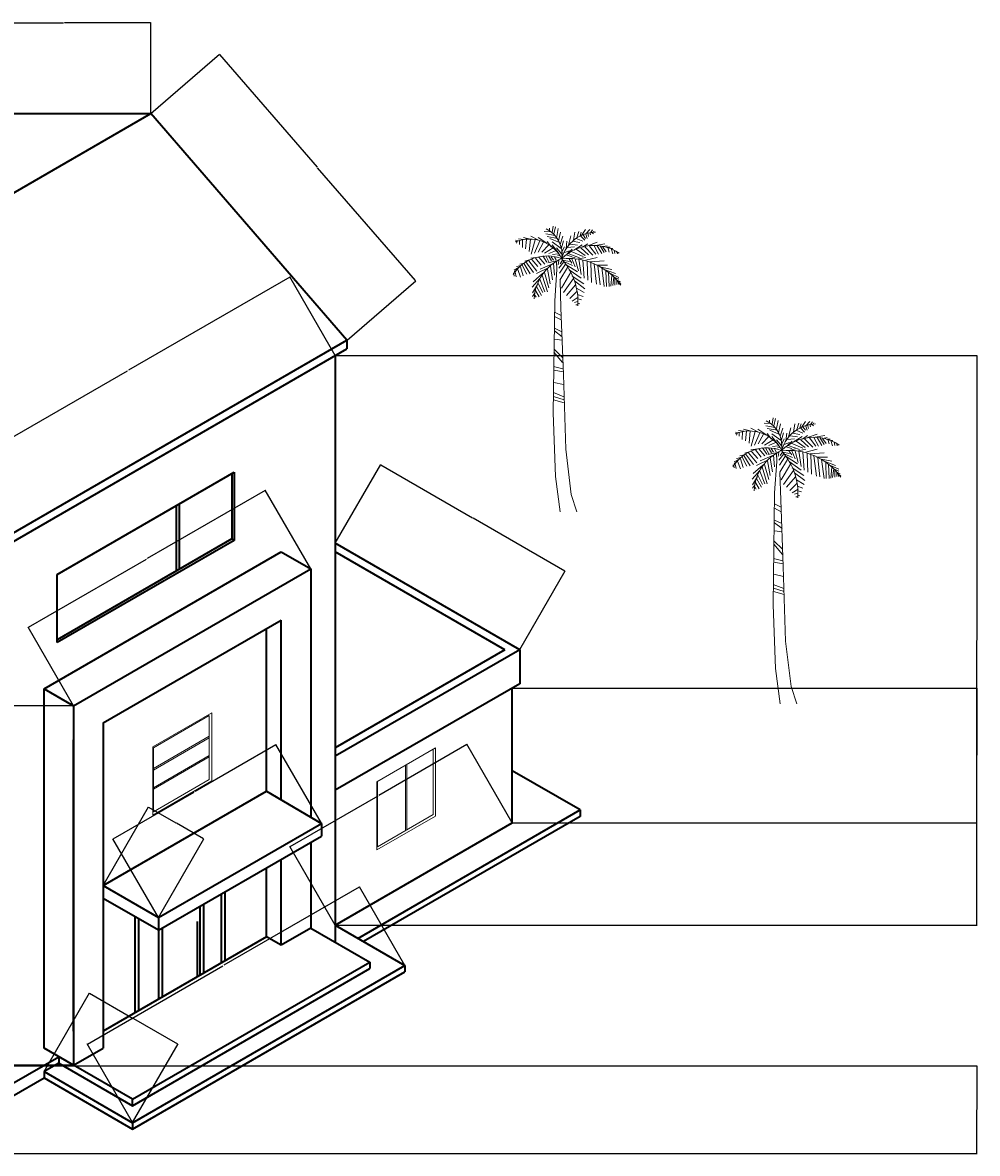
# Model space of a CAD drawing. Units: inches. Extents: x 159268 to 319465, y 115871 to 232488.
# Tile 2 of 2: x 159989 to 160662, y 116007 to 116803. Entities that reach past the tile are written whole.
import ezdxf

# ---------------------------------------------------------------- set-up
doc = ezdxf.new("R2010")
doc.units = ezdxf.units.IN
for name, color, linetype, lineweight in [('A-ANNO-DIMS', 2, 'Continuous', 18), ('A-ELEV', 7, 'Continuous', 35), ('A-GLAZ', 4, 'Continuous', 18), ('L-PLNT', 3, 'Continuous', 13)]:
    doc.layers.add(name, color=color, linetype=linetype, lineweight=lineweight)
doc.styles.get("Standard").update_dxf_attribs({"font": 'arial.ttf'})
doc.dimstyles.get("Standard").update_dxf_attribs({"dimtxt": 0.18, "dimasz": 0.18, "dimexe": 0.18, "dimexo": 0.0625, "dimgap": 0.09, "dimtad": 0, "dimtih": 1, "dimtoh": 1, "dimdec": 4, "dimzin": 0, "dimdsep": 46, "dimtxsty": 'Standard', "dimcen": 0.09, "dimadec": 0, "dimazin": 0, "dimtfac": 1, "dimtdec": 4, "dimtofl": 0, "dimtmove": 0, "dimatfit": 3, "dimfxl": 1, "dimtolj": 1, "dimtzin": 0, "dimarcsym": 0})

# ---------------------------------------------------------------- blocks, each defined once
blk = doc.blocks.new('*U5')
for p, q in [((-7.5, 199.68), (-7.5, 197.946)), ((-5.567, 196.707), (-4.987, 201.167)), ((-4.407, 195.716), (-3.247, 200.672)), ((-2.474, 193.733), (-1.315, 199.433)), ((-29.729, 190.759), (-31.469, 191.255)), ((-25.283, 191.751), (-29.342, 192.246)), ((-26.443, 191.503), (-26.636, 186.051)), ((-20.064, 191.751), (-25.863, 193.238)), ((-23.737, 191.751), (-24.51, 185.06)), ((-21.031, 191.998), (-21.804, 183.325)), ((-15.232, 191.255), (-20.644, 193.981)), ((-17.551, 191.503), (-20.451, 181.343)), ((-9.433, 189.025), (-15.618, 193.238)), ((-6.727, 197.202), (-11.366, 197.45)), ((-3.441, 194.477), (-10.013, 195.716)), ((-1.894, 192.494), (-9.24, 193.733)), ((-0.541, 189.52), (-7.307, 192.494)), ((-1.121, 190.759), (0.232, 196.955)), ((0.038, 188.281), (1.778, 193.981)), ((5.837, 187.786), (7.577, 194.229)), ((9.317, 191.255), (10.283, 196.955)), ((11.25, 192.494), (15.889, 190.512)), ((11.829, 192.99), (13.182, 197.45)), ((13.956, 194.229), (14.729, 196.955)), ((14.536, 193.981), (17.242, 191.255)), ((15.116, 194.477), (17.822, 198.689)), ((16.082, 194.972), (17.822, 192.494)), ((18.015, 195.716), (20.914, 198.689)), ((18.015, 195.468), (18.981, 192.494)), ((19.368, 196.459), (19.948, 193.733)), ((20.914, 196.459), (21.301, 194.972)), ((21.301, 196.459), (22.847, 198.441)), ((22.074, 196.707), (23.427, 195.716)), ((23.234, 196.707), (23.62, 197.698)), ((-30.309, 190.512), (-30.695, 189.025)), ((-28.763, 190.759), (-28.763, 188.281)), ((-14.265, 190.759), (-18.131, 182.086)), ((-11.753, 189.768), (-15.425, 182.83)), ((-8.08, 188.034), (-12.912, 182.83)), ((-4.987, 185.803), (-10.979, 182.086)), ((-6.147, 186.299), (-9.24, 190.264)), ((-3.247, 183.821), (-8.08, 181.838)), ((-5.76, 190.016), (0.618, 185.308)), ((-5.76, 188.034), (-1.508, 182.582)), ((-2.668, 185.803), (1.198, 181.343)), ((1.005, 185.803), (2.358, 190.759)), ((1.005, 182.582), (2.938, 186.547)), ((2.938, 182.582), (6.61, 183.821)), ((4.098, 185.06), (4.678, 190.512)), ((4.871, 186.051), (10.09, 186.547)), ((4.871, 181.591), (8.544, 184.812)), ((6.997, 188.529), (12.216, 187.786)), ((7.77, 183.325), (16.082, 179.856)), ((8.544, 190.512), (13.763, 189.52)), ((9.51, 184.317), (15.502, 188.034)), ((11.25, 184.812), (17.628, 180.352)), ((14.536, 185.803), (19.948, 180.847)), ((15.695, 186.299), (19.368, 188.777)), ((17.242, 186.547), (23.041, 180.599)), ((19.368, 187.29), (26.133, 189.768)), ((20.721, 187.042), (25.167, 181.343)), ((23.814, 187.29), (26.907, 181.343)), ((24.78, 187.538), (31.546, 188.777)), ((26.133, 187.29), (29.419, 181.838)), ((28.066, 187.29), (30.966, 182.582)), ((29.806, 186.795), (32.319, 183.078)), ((29.999, 186.795), (33.092, 187.29)), ((32.512, 186.299), (35.218, 186.299)), ((33.479, 186.051), (34.445, 182.83)), ((35.605, 185.556), (37.151, 185.308)), ((35.798, 185.308), (36.958, 181.591)), ((38.118, 184.317), (38.504, 181.838)), ((-25.09, 175.148), (-28.376, 174.404)), ((-21.031, 177.626), (-24.897, 176.387)), ((-24.317, 175.891), (-18.711, 168.457)), ((-22.191, 176.635), (-16.391, 169.448)), ((-15.618, 179.36), (-20.644, 178.617)), ((-20.064, 177.626), (-15.812, 172.67)), ((-17.358, 178.617), (-13.299, 173.661)), ((-15.038, 179.36), (-10.786, 174.404)), ((-4.214, 175.148), (-14.072, 170.935)), ((-12.332, 180.104), (-9.433, 175.643)), ((-10.206, 180.104), (-8.08, 175.891)), ((-1.701, 176.882), (-8.66, 175.396)), ((-8.273, 180.104), (-6.147, 176.635)), ((-6.34, 179.608), (-4.6, 177.13)), ((-1.315, 181.591), (-5.374, 181.095)), ((-4.021, 179.36), (-2.861, 177.378)), ((-2.668, 176.387), (-2.376, 170.594)), ((-0.348, 180.352), (-1.894, 180.104)), ((-0.928, 176.882), (-1.508, 173.909)), ((2.551, 175.891), (-0.928, 171.431)), ((1.585, 177.13), (0.038, 174.652)), ((1.585, 177.13), (6.61, 176.139)), ((2.938, 175.891), (8.737, 173.413)), ((4.098, 180.847), (8.35, 179.608)), ((5.644, 181.838), (13.569, 178.865)), ((6.224, 178.121), (8.157, 175.148)), ((7.384, 178.369), (10.476, 179.36)), ((8.157, 178.121), (10.476, 172.422)), ((10.476, 177.874), (12.796, 169.696)), ((11.829, 177.874), (18.015, 179.113)), ((13.182, 177.874), (14.729, 166.97)), ((15.889, 177.13), (16.855, 164.492)), ((18.015, 177.13), (26.133, 179.113)), ((18.981, 175.891), (19.561, 163.005)), ((20.914, 175.891), (30.966, 176.635)), ((21.688, 175.396), (22.074, 161.518)), ((39.857, 182.83), (40.244, 181.591)), ((-32.628, 167.961), (-33.208, 167.961)), ((-32.628, 167.713), (-32.435, 165.979)), ((-28.956, 172.174), (-32.435, 170.192)), ((-31.082, 169.944), (-32.435, 169.2)), ((-31.662, 168.705), (-31.082, 165.483)), ((-27.409, 173.413), (-30.695, 172.67)), ((-29.922, 170.687), (-27.989, 165.235)), ((-27.989, 172.422), (-26.056, 166.227)), ((-26.829, 173.661), (-23.544, 167.218)), ((-25.476, 174.652), (-21.224, 167.466)), ((-12.139, 167.961), (-19.098, 162.014)), ((-8.466, 171.678), (-16.585, 167.713)), ((-10.979, 168.457), (-7.887, 157.801)), ((-8.853, 170.935), (-7.113, 160.527)), ((-6.92, 172.917), (-5.374, 163.253)), ((-4.6, 174.9), (-4.021, 166.722)), ((3.711, 174.404), (-0.541, 167.961)), ((5.257, 171.926), (-0.155, 163.005)), ((7.384, 168.705), (0.812, 157.553)), ((4.291, 173.909), (12.216, 168.953)), ((6.417, 170.439), (14.729, 164.492)), ((23.814, 174.404), (25.554, 160.279)), ((25.554, 173.661), (33.285, 173.661)), ((26.52, 173.165), (28.066, 159.784)), ((28.839, 172.174), (36.378, 170.687)), ((29.226, 171.926), (30.966, 158.545)), ((30.966, 170.687), (38.891, 167.713)), ((32.126, 169.696), (32.512, 158.545)), ((34.058, 168.705), (34.445, 158.545)), ((35.412, 167.713), (41.404, 164.988)), ((-14.265, 164.244), (-19.678, 158.049)), ((-16.005, 160.031), (-19.484, 154.084)), ((-15.618, 160.775), (-12.332, 154.332)), ((-14.265, 163.749), (-10.786, 154.828)), ((-12.719, 166.722), (-9.046, 154.828)), ((9.317, 164.244), (2.358, 154.332)), ((10.863, 159.784), (4.484, 152.35)), ((8.544, 165.979), (16.662, 160.527)), ((10.09, 162.51), (17.435, 157.058)), ((36.378, 166.474), (35.605, 158.792)), ((37.731, 165.235), (36.958, 159.288)), ((37.924, 165.235), (41.404, 163.749)), ((38.504, 164.492), (38.504, 159.536)), ((39.664, 163.253), (42.37, 161.766)), ((39.857, 162.757), (39.857, 160.031)), ((40.824, 161.766), (41.21, 160.031)), ((41.21, 161.518), (42.757, 160.279)), ((-18.131, 153.589), (-19.484, 151.606)), ((-17.938, 152.597), (-16.972, 151.111)), ((-17.358, 155.819), (-14.845, 151.358)), ((-16.585, 158.545), (-13.106, 152.35)), ((11.829, 155.075), (6.804, 150.119)), ((11.443, 157.553), (16.855, 154.332)), ((12.216, 153.093), (16.082, 151.606)), ((12.603, 151.111), (8.544, 148.385)), ((12.216, 148.137), (10.09, 147.393)), ((12.409, 145.659), (11.056, 145.659)), ((12.409, 146.898), (13.763, 146.402)), ((12.603, 149.872), (15.116, 149.128)), ((-4.081, 140.645), (0.753, 138.261)), ((-4.081, 137.547), (0.753, 135.163)), ((-4.081, 129.205), (1.124, 126.821)), ((-4.081, 127.298), (1.31, 123.246)), ((-4.081, 121.578), (1.31, 120.863)), ((-4.453, 112.283), (1.682, 105.133)), ((-4.267, 114.428), (1.682, 108.708)), ((-4.639, 102.273), (1.868, 100.604)), ((-4.453, 99.651), (2.24, 98.459)), ((-4.453, 91.071), (2.426, 89.641)), ((-4.825, 83.921), (2.612, 81.061)), ((-4.639, 81.299), (2.797, 78.916)), ((-4.639, 78.916), (2.797, 76.771))]:
    blk.add_line(p, q)
for points in [[(-2.363, 170.553), (-3.88, 148.505), (-4.988, 69.634), (-3.325, 24.869), (0, 0)], [(-0.116, 162.848), (0.554, 143.532), (2.217, 96.635), (3.88, 44.054), (7.76, 12.079), (11.64, 0)]]:
    blk.add_lwpolyline(points)
for centre, radius, start, end in [((-18.427, 181.448), 19.715, 350.285, 64.11229), ((-21.738, 166.094), 25.899, 27.67115, 112.5305), ((25.595, 171.567), 25.395, 91.40319, 163.882), ((23.687, 155.341), 32.188, 56.19272, 134.3213), ((-9.259, 151.732), 28.386, 68.38311, 147.5322), ((14.394, 148.393), 32.752, 113.7592, 177.4133), ((5.828, 132.718), 45.639, 35.98777, 95.82273), ((-32.8, 147.923), 45.309, 356.1943, 41.37848)]:
    blk.add_arc(centre, radius, start, end)
blk = doc.blocks.new('*D19')
at = {"layer": 'A-ANNO-DIMS', "color": 0, "lineweight": -2, "transparency": 16777216}
for p, q in [((159822.54, 116068.59), (160661.48, 116068.59)), ((160661.3, 116068.41), (160661.3, 116037.95)), ((160661.3, 116007.12), (160661.3, 116037.59)), ((159822.54, 116006.94), (160661.48, 116006.94))]:
    blk.add_line(p, q, dxfattribs=at)
at = {"layer": 'A-ANNO-DIMS', "color": 0, "transparency": 16777216}
for points in [[(160661.27, 116068.41), (160661.33, 116068.41), (160661.3, 116068.59)], [(160661.27, 116007.12), (160661.33, 116007.12), (160661.3, 116006.94)]]:
    blk.add_solid(points, dxfattribs=at)
at = {"layer": 'Defpoints', "color": 0, "transparency": 16777216}
for p in [(159822.48, 116068.59), (160661.3, 116068.59), (159822.48, 116006.94)]:
    blk.add_point(p, dxfattribs=at)
at = {"layer": 'A-ANNO-DIMS', "color": 0, "transparency": 16777216, "insert": (160661.3, 116037.77), "char_height": 0.18, "attachment_point": 5}
blk.add_mtext('\\A1;61.65', dxfattribs=at)
blk = doc.blocks.new('*D20')
at = {"layer": 'A-ANNO-DIMS', "color": 0, "lineweight": -2, "transparency": 16777216}
for p, q in [((160177.25, 116623.87), (160063.72, 116558.33)), ((160209.3, 116568.72), (160177.32, 116624.12)), ((159949.55, 116492.41), (160063.09, 116557.96)), ((159981.29, 116437.08), (159949.31, 116492.48))]:
    blk.add_line(p, q, dxfattribs=at)
at = {"layer": 'A-ANNO-DIMS', "color": 0, "transparency": 16777216}
for points in [[(160177.23, 116623.9), (160177.26, 116623.85), (160177.41, 116623.96)], [(159949.54, 116492.44), (159949.57, 116492.39), (159949.4, 116492.32)]]:
    blk.add_solid(points, dxfattribs=at)
at = {"layer": 'Defpoints', "color": 0, "transparency": 16777216}
for p in [(160177.41, 116623.96), (160209.33, 116568.67), (159981.32, 116437.03)]:
    blk.add_point(p, dxfattribs=at)
at = {"layer": 'A-ANNO-DIMS', "color": 0, "transparency": 16777216, "insert": (160063.4, 116558.14), "char_height": 0.18, "attachment_point": 5}
blk.add_mtext('\\A1;263.3', dxfattribs=at)
blk = doc.blocks.new('*D21')
at = {"layer": 'A-ANNO-DIMS', "color": 0, "lineweight": -2, "transparency": 16777216}
for p, q in [((160209.39, 116568.67), (160661.48, 116568.67)), ((160661.3, 116568.49), (160661.3, 116368.29)), ((160661.3, 116167.73), (160661.3, 116367.93)), ((160209.39, 116167.55), (160661.48, 116167.55))]:
    blk.add_line(p, q, dxfattribs=at)
at = {"layer": 'A-ANNO-DIMS', "color": 0, "transparency": 16777216}
for points in [[(160661.27, 116568.49), (160661.33, 116568.49), (160661.3, 116568.67)], [(160661.27, 116167.73), (160661.33, 116167.73), (160661.3, 116167.55)]]:
    blk.add_solid(points, dxfattribs=at)
at = {"layer": 'Defpoints', "color": 0, "transparency": 16777216}
for p in [(160209.33, 116568.67), (160661.3, 116568.67), (160209.33, 116167.55)]:
    blk.add_point(p, dxfattribs=at)
at = {"layer": 'A-ANNO-DIMS', "color": 0, "transparency": 16777216, "insert": (160661.3, 116368.11), "char_height": 0.18, "attachment_point": 5}
blk.add_mtext('\\A1;401.1', dxfattribs=at)
blk = doc.blocks.new('*D22')
at = {"layer": 'A-ANNO-DIMS', "color": 0, "lineweight": -2, "transparency": 16777216}
for p, q in [((160024.97, 116321.98), (159267.73, 116321.98)), ((159267.91, 116321.8), (159267.91, 116195.69)), ((159267.91, 116069.21), (159267.91, 116195.33)), ((160024.97, 116069.03), (159267.73, 116069.03))]:
    blk.add_line(p, q, dxfattribs=at)
at = {"layer": 'A-ANNO-DIMS', "color": 0, "transparency": 16777216}
for points in [[(159267.88, 116321.8), (159267.94, 116321.8), (159267.91, 116321.98)], [(159267.88, 116069.21), (159267.94, 116069.21), (159267.91, 116069.03)]]:
    blk.add_solid(points, dxfattribs=at)
at = {"layer": 'Defpoints', "color": 0, "transparency": 16777216}
for p in [(159267.91, 116321.98), (160025.03, 116321.98), (160025.03, 116069.03)]:
    blk.add_point(p, dxfattribs=at)
at = {"layer": 'A-ANNO-DIMS', "color": 0, "transparency": 16777216, "insert": (159267.91, 116195.51), "char_height": 0.18, "attachment_point": 5}
blk.add_mtext('\\A1;252.95', dxfattribs=at)
blk = doc.blocks.new('*D23')
at = {"layer": 'A-ANNO-DIMS', "color": 0, "lineweight": -2, "transparency": 16777216}
for p, q in [((160160.03, 116473.65), (160076.96, 116425.69)), ((160192.08, 116418.5), (160160.1, 116473.9)), ((159993.26, 116377.37), (160076.33, 116425.33)), ((160025, 116322.04), (159993.02, 116377.44))]:
    blk.add_line(p, q, dxfattribs=at)
at = {"layer": 'A-ANNO-DIMS', "color": 0, "transparency": 16777216}
for points in [[(160160.01, 116473.68), (160160.04, 116473.63), (160160.19, 116473.74)], [(159993.25, 116377.4), (159993.28, 116377.34), (159993.11, 116377.28)]]:
    blk.add_solid(points, dxfattribs=at)
at = {"layer": 'Defpoints', "color": 0, "transparency": 16777216}
for p in [(160160.19, 116473.74), (160192.11, 116418.45), (160025.03, 116321.98)]:
    blk.add_point(p, dxfattribs=at)
at = {"layer": 'A-ANNO-DIMS', "color": 0, "transparency": 16777216, "insert": (160076.65, 116425.51), "char_height": 0.18, "attachment_point": 5}
blk.add_mtext('\\A1;192.93', dxfattribs=at)
blk = doc.blocks.new('*D24')
at = {"layer": 'A-ANNO-DIMS', "color": 0, "lineweight": -2, "transparency": 16777216}
for p, q in [((160167.52, 116294.5), (160110.58, 116261.63)), ((160199.57, 116239.35), (160167.59, 116294.75)), ((160053.02, 116228.39), (160109.95, 116261.27)), ((160084.76, 116173.06), (160052.77, 116228.46))]:
    blk.add_line(p, q, dxfattribs=at)
at = {"layer": 'A-ANNO-DIMS', "color": 0, "transparency": 16777216}
for points in [[(160167.51, 116294.53), (160167.54, 116294.48), (160167.68, 116294.59)], [(160053, 116228.42), (160053.03, 116228.37), (160052.86, 116228.3)]]:
    blk.add_solid(points, dxfattribs=at)
at = {"layer": 'Defpoints', "color": 0, "transparency": 16777216}
for p in [(160167.68, 116294.59), (160199.6, 116239.3), (160084.79, 116173.01)]:
    blk.add_point(p, dxfattribs=at)
at = {"layer": 'A-ANNO-DIMS', "color": 0, "transparency": 16777216, "insert": (160110.27, 116261.45), "char_height": 0.18, "attachment_point": 5}
blk.add_mtext('\\A1;132.58', dxfattribs=at)
blk = doc.blocks.new('*D25')
at = {"layer": 'A-ANNO-DIMS', "color": 0, "lineweight": -2, "transparency": 16777216}
for p, q in [((160045.85, 116195.56), (160077.83, 116250.96)), ((160077.9, 116250.71), (160097, 116239.68)), ((160116.56, 116228.39), (160097.45, 116239.43)), ((160084.82, 116173.06), (160116.8, 116228.46))]:
    blk.add_line(p, q, dxfattribs=at)
at = {"layer": 'A-ANNO-DIMS', "color": 0, "transparency": 16777216}
for points in [[(160077.91, 116250.74), (160077.88, 116250.69), (160077.74, 116250.8)], [(160116.57, 116228.42), (160116.54, 116228.37), (160116.71, 116228.3)]]:
    blk.add_solid(points, dxfattribs=at)
at = {"layer": 'Defpoints', "color": 0, "transparency": 16777216}
for p in [(160116.71, 116228.3), (160045.82, 116195.51), (160084.79, 116173.01)]:
    blk.add_point(p, dxfattribs=at)
at = {"layer": 'A-ANNO-DIMS', "color": 0, "transparency": 16777216, "insert": (160097.23, 116239.55), "char_height": 0.18, "attachment_point": 5}
blk.add_mtext('\\A1;45', dxfattribs=at)
blk = doc.blocks.new('*D26')
at = {"layer": 'A-ANNO-DIMS', "color": 0, "lineweight": -2, "transparency": 16777216}
for p, q in [((160226.28, 116194.45), (160130.87, 116139.37)), ((160258.33, 116139.3), (160226.35, 116194.7)), ((160034.83, 116083.92), (160130.24, 116139)), ((160066.57, 116028.59), (160034.59, 116083.98))]:
    blk.add_line(p, q, dxfattribs=at)
at = {"layer": 'A-ANNO-DIMS', "color": 0, "transparency": 16777216}
for points in [[(160226.26, 116194.48), (160226.29, 116194.43), (160226.44, 116194.54)], [(160034.82, 116083.94), (160034.85, 116083.89), (160034.68, 116083.83)]]:
    blk.add_solid(points, dxfattribs=at)
at = {"layer": 'Defpoints', "color": 0, "transparency": 16777216}
for p in [(160226.44, 116194.54), (160258.36, 116139.25), (160066.6, 116028.53)]:
    blk.add_point(p, dxfattribs=at)
at = {"layer": 'A-ANNO-DIMS', "color": 0, "transparency": 16777216, "insert": (160130.56, 116139.18), "char_height": 0.18, "attachment_point": 5}
blk.add_mtext('\\A1;221.43', dxfattribs=at)
blk = doc.blocks.new('*D27')
at = {"layer": 'A-ANNO-DIMS', "color": 0, "lineweight": -2, "transparency": 16777216}
for p, q in [((160004.28, 116064.59), (160036.26, 116119.98)), ((160036.33, 116119.74), (160067.13, 116101.95)), ((160098.37, 116083.92), (160067.57, 116101.7)), ((160066.63, 116028.59), (160098.62, 116083.98))]:
    blk.add_line(p, q, dxfattribs=at)
at = {"layer": 'A-ANNO-DIMS', "color": 0, "transparency": 16777216}
for points in [[(160036.34, 116119.76), (160036.31, 116119.71), (160036.17, 116119.83)], [(160098.38, 116083.94), (160098.35, 116083.89), (160098.53, 116083.83)]]:
    blk.add_solid(points, dxfattribs=at)
at = {"layer": 'Defpoints', "color": 0, "transparency": 16777216}
for p in [(160098.53, 116083.83), (160004.25, 116064.53), (160066.6, 116028.53)]:
    blk.add_point(p, dxfattribs=at)
at = {"layer": 'A-ANNO-DIMS', "color": 0, "transparency": 16777216, "insert": (160067.35, 116101.83), "char_height": 0.18, "attachment_point": 5}
blk.add_mtext('\\A1;72', dxfattribs=at)
blk = doc.blocks.new('*D28')
at = {"layer": 'A-ANNO-DIMS', "color": 0, "lineweight": -2, "transparency": 16777216}
for p, q in [((160334.01, 116239.61), (160302.02, 116295)), ((160301.96, 116294.76), (160240.04, 116259.01)), ((160177.56, 116222.94), (160239.48, 116258.69)), ((160209.3, 116167.61), (160177.32, 116223))]:
    blk.add_line(p, q, dxfattribs=at)
at = {"layer": 'A-ANNO-DIMS', "color": 0, "transparency": 16777216}
for points in [[(160301.94, 116294.78), (160301.97, 116294.73), (160302.11, 116294.85)], [(160177.55, 116222.96), (160177.58, 116222.91), (160177.41, 116222.85)]]:
    blk.add_solid(points, dxfattribs=at)
at = {"layer": 'Defpoints', "color": 0, "transparency": 16777216}
for p in [(160302.11, 116294.85), (160334.04, 116239.55), (160209.33, 116167.55)]:
    blk.add_point(p, dxfattribs=at)
at = {"layer": 'A-ANNO-DIMS', "color": 0, "transparency": 16777216, "insert": (160239.76, 116258.85), "char_height": 0.18, "attachment_point": 5}
blk.add_mtext('\\A1;144', dxfattribs=at)
blk = doc.blocks.new('*D29')
at = {"layer": 'A-ANNO-DIMS', "color": 0, "lineweight": -2, "transparency": 16777216}
for p, q in [((160209.36, 116436.61), (160241.35, 116492)), ((160241.41, 116491.76), (160305.93, 116454.51)), ((160371, 116416.94), (160306.49, 116454.19)), ((160339.27, 116361.61), (160371.25, 116417))]:
    blk.add_line(p, q, dxfattribs=at)
at = {"layer": 'A-ANNO-DIMS', "color": 0, "transparency": 16777216}
for points in [[(160241.43, 116491.78), (160241.4, 116491.73), (160241.26, 116491.85)], [(160371.02, 116416.96), (160370.99, 116416.91), (160371.16, 116416.85)]]:
    blk.add_solid(points, dxfattribs=at)
at = {"layer": 'Defpoints', "color": 0, "transparency": 16777216}
for p in [(160209.33, 116436.55), (160371.16, 116416.85), (160339.23, 116361.55)]:
    blk.add_point(p, dxfattribs=at)
at = {"layer": 'A-ANNO-DIMS', "color": 0, "transparency": 16777216, "insert": (160306.21, 116454.35), "char_height": 0.18, "attachment_point": 5}
blk.add_mtext('\\A1;150', dxfattribs=at)
blk = doc.blocks.new('*D30')
at = {"layer": 'A-ANNO-DIMS', "color": 0, "lineweight": -2, "transparency": 16777216}
for p, q in [((160334.1, 116334.55), (160661.48, 116334.55)), ((160661.3, 116334.37), (160661.3, 116287.23)), ((160661.3, 116239.73), (160661.3, 116286.87)), ((160334.1, 116239.55), (160661.48, 116239.55))]:
    blk.add_line(p, q, dxfattribs=at)
at = {"layer": 'A-ANNO-DIMS', "color": 0, "transparency": 16777216}
for points in [[(160661.27, 116334.37), (160661.33, 116334.37), (160661.3, 116334.55)], [(160661.27, 116239.73), (160661.33, 116239.73), (160661.3, 116239.55)]]:
    blk.add_solid(points, dxfattribs=at)
at = {"layer": 'Defpoints', "color": 0, "transparency": 16777216}
for p in [(160334.04, 116334.55), (160661.3, 116334.55), (160334.04, 116239.55)]:
    blk.add_point(p, dxfattribs=at)
at = {"layer": 'A-ANNO-DIMS', "color": 0, "transparency": 16777216, "insert": (160661.3, 116287.05), "char_height": 0.18, "attachment_point": 5}
blk.add_mtext('\\A1;95', dxfattribs=at)
blk = doc.blocks.new('*D34')
at = {"layer": 'A-ANNO-DIMS', "color": 0, "lineweight": -2, "transparency": 16777216}
for p, q in [((159957.3, 116739.08), (159957.3, 116803.05)), ((159957.48, 116802.87), (160017.98, 116802.87)), ((160079.23, 116802.87), (160018.72, 116802.87)), ((160079.41, 116739.08), (160079.41, 116803.05))]:
    blk.add_line(p, q, dxfattribs=at)
at = {"layer": 'A-ANNO-DIMS', "color": 0, "transparency": 16777216}
for points in [[(159957.48, 116802.9), (159957.48, 116802.84), (159957.3, 116802.87)], [(160079.23, 116802.9), (160079.23, 116802.84), (160079.41, 116802.87)]]:
    blk.add_solid(points, dxfattribs=at)
at = {"layer": 'Defpoints', "color": 0, "transparency": 16777216}
for p in [(160079.41, 116802.87), (159957.3, 116739.02), (160079.41, 116739.02)]:
    blk.add_point(p, dxfattribs=at)
at = {"layer": 'A-ANNO-DIMS', "color": 0, "transparency": 16777216, "insert": (160018.35, 116802.87), "char_height": 0.18, "attachment_point": 5}
blk.add_mtext('\\A1;122.1', dxfattribs=at)
blk = doc.blocks.new('*D35')
at = {"layer": 'A-ANNO-DIMS', "color": 0, "lineweight": -2, "transparency": 16777216}
for p, q in [((160079.45, 116739.06), (160127.81, 116780.94)), ((160127.79, 116780.68), (160196.61, 116701.21)), ((160265.75, 116621.38), (160196.93, 116700.85)), ((160217.65, 116579.48), (160266, 116621.36))]:
    blk.add_line(p, q, dxfattribs=at)
at = {"layer": 'A-ANNO-DIMS', "color": 0, "transparency": 16777216}
for points in [[(160127.81, 116780.7), (160127.77, 116780.66), (160127.67, 116780.82)], [(160265.77, 116621.4), (160265.73, 116621.36), (160265.87, 116621.24)]]:
    blk.add_solid(points, dxfattribs=at)
at = {"layer": 'Defpoints', "color": 0, "transparency": 16777216}
for p in [(160079.41, 116739.02), (160265.87, 116621.24), (160217.6, 116579.44)]:
    blk.add_point(p, dxfattribs=at)
at = {"layer": 'A-ANNO-DIMS', "color": 0, "transparency": 16777216, "insert": (160196.77, 116701.03), "char_height": 0.18, "attachment_point": 5}
blk.add_mtext('\\A1;211.1', dxfattribs=at)

msp = doc.modelspace()

# ---------------------------------------------------------------- linework, layer by layer
at = {"layer": 'A-ELEV'}
for p, q in [((159819.109, 116588.735), (160079.407, 116739.018)), ((159957.297, 116739.018), (160079.407, 116739.018)), ((160217.603, 116579.444), (160079.407, 116739.018)), ((159957.305, 116429.161), (160217.603, 116579.444)), ((160217.603, 116579.444), (160217.603, 116573.444)), ((159957.305, 116423.161), (160217.603, 116573.444)), ((160209.331, 116568.668), (160209.331, 116452.39)), ((160013.556, 116414.547), (160138.264, 116486.547)), ((160138.264, 116486.547), (160138.264, 116438.547)), ((160136.496, 116485.611), (160136.496, 116439.527)), ((160097.187, 116462.832), (160097.187, 116416.832)), ((160099.425, 116464.124), (160099.425, 116418.124)), ((160209.331, 116452.39), (160209.331, 116155.553)), ((160136.496, 116439.527), (160013.556, 116368.547)), ((160138.264, 116438.547), (160013.556, 116366.547)), ((160136.496, 116439.527), (160138.229, 116438.527)), ((160004.247, 116333.984), (160171.326, 116430.447)), ((160171.326, 116430.447), (160192.11, 116418.447)), ((160339.234, 116361.553), (160209.331, 116436.553)), ((160328.842, 116361.553), (160209.331, 116430.553)), ((160013.556, 116366.547), (160013.556, 116414.547)), ((160025.031, 116321.984), (160192.11, 116418.447)), ((160192.11, 116418.447), (160192.11, 116243.971)), ((160045.816, 116309.984), (160171.326, 116382.447)), ((160160.933, 116261.971), (160160.933, 116376.447)), ((160171.325, 116255.971), (160171.326, 116382.447)), ((160328.842, 116361.553), (160209.331, 116292.553)), ((160339.234, 116361.553), (160209.331, 116286.553)), ((160339.234, 116361.553), (160339.234, 116337.553)), ((160339.234, 116337.553), (160209.331, 116262.553)), ((160004.247, 116081.033), (160004.247, 116333.984)), ((160004.247, 116333.984), (160025.031, 116321.984)), ((160334.038, 116239.553), (160334.038, 116334.553)), ((160025.031, 116321.984), (160025.031, 116069.033)), ((160045.816, 116309.984), (160045.816, 116081.033)), ((160025.031, 116093.033), (160025.031, 116297.984)), ((160381.825, 116248.728), (160334.038, 116276.318)), ((160045.816, 116195.509), (160160.933, 116261.971)), ((160160.933, 116261.971), (160199.602, 116239.297)), ((160225.278, 116158.346), (160381.825, 116248.728)), ((160381.825, 116248.728), (160381.825, 116244.228)), ((160084.787, 116173.009), (160199.602, 116239.297)), ((160199.602, 116239.297), (160199.602, 116230.297)), ((160209.331, 116167.553), (160334.038, 116239.553)), ((160381.825, 116244.228), (160229.175, 116156.096)), ((160084.787, 116164.009), (160199.602, 116230.297)), ((160192.11, 116225.971), (160192.109, 116165.495)), ((160160.932, 116159.495), (160160.933, 116207.971)), ((160171.325, 116153.495), (160171.325, 116213.971)), ((160045.816, 116195.509), (160084.787, 116173.009)), ((160084.787, 116164.009), (160045.816, 116186.509)), ((160129.255, 116141.206), (160129.255, 116189.682)), ((160131.853, 116142.706), (160131.853, 116191.182)), ((160113.982, 116180.864), (160113.982, 116132.388)), ((160116.58, 116182.364), (160116.58, 116133.888)), ((160068.261, 116173.55), (160068.261, 116105.991)), ((160070.859, 116172.05), (160070.859, 116107.491)), ((160084.787, 116173.009), (160084.787, 116164.009)), ((160112.141, 116170.112), (160112.141, 116131.429)), ((160084.787, 116164.009), (160084.787, 116115.533)), ((160087.385, 116165.509), (160087.385, 116117.033)), ((160192.109, 116165.495), (160171.325, 116153.495)), ((160192.109, 116165.495), (160233.679, 116141.495)), ((160209.331, 116167.553), (160258.36, 116139.245)), ((160160.932, 116159.495), (160045.816, 116093.033)), ((160171.325, 116153.495), (160160.932, 116159.495)), ((160066.601, 116045.033), (160233.679, 116141.495)), ((160066.601, 116028.533), (160258.36, 116139.245)), ((160066.601, 116040.533), (160233.679, 116136.995)), ((160233.679, 116141.495), (160233.679, 116136.995)), ((160258.36, 116139.245), (160258.36, 116134.745)), ((160066.601, 116024.033), (160258.36, 116134.745)), ((160025.031, 116069.033), (160004.247, 116081.033)), ((160025.031, 116069.033), (160045.816, 116081.033)), ((159981.532, 116055.918), (160014.639, 116075.033)), ((160014.639, 116075.033), (160014.639, 116070.533)), ((160014.639, 116070.533), (160004.247, 116064.533)), ((160004.247, 116064.533), (160066.601, 116028.533)), ((160004.247, 116064.533), (160004.247, 116060.033)), ((160014.639, 116070.533), (160066.601, 116040.533)), ((160066.601, 116045.033), (160025.031, 116069.033)), ((159981.532, 116046.918), (160004.247, 116060.033)), ((160004.247, 116060.033), (160066.601, 116024.033)), ((160066.601, 116040.533), (160066.601, 116045.033)), ((160066.601, 116028.533), (160066.601, 116024.033))]:
    msp.add_line(p, q, dxfattribs=at)
at = {"layer": 'A-GLAZ'}
for p, q in [((160080.819, 116293.149), (160122.388, 116317.149)), ((160081.252, 116292.399), (160120.656, 116315.149)), ((160120.656, 116315.149), (160120.656, 116270.149)), ((160122.388, 116317.149), (160122.388, 116269.149)), ((160081.252, 116277.842), (160120.656, 116300.592)), ((160081.252, 116276.842), (160120.656, 116299.592)), ((160080.819, 116245.149), (160080.819, 116293.149)), ((160081.252, 116247.399), (160081.252, 116292.399)), ((160081.252, 116264.327), (160120.656, 116287.077)), ((160238.564, 116268.565), (160279.962, 116292.466)), ((160278.23, 116291.466), (160278.23, 116245.466)), ((160279.962, 116292.466), (160279.962, 116244.466)), ((160081.252, 116263.327), (160120.656, 116286.077)), ((160258.83, 116280.265), (160258.83, 116234.265)), ((160259.696, 116280.765), (160259.696, 116234.765)), ((160122.388, 116269.149), (160080.819, 116245.149)), ((160120.656, 116270.149), (160081.252, 116247.399)), ((160238.564, 116220.565), (160238.564, 116268.565)), ((160238.997, 116222.815), (160238.997, 116268.815)), ((160238.564, 116220.565), (160279.962, 116244.466)), ((160238.997, 116222.815), (160278.23, 116245.466))]:
    msp.add_line(p, q, dxfattribs=at)

# ---------------------------------------------------------------- block references
at = {"layer": 'L-PLNT'}
for p in [(160367.776, 116458.636), (160522.684, 116323.56)]:
    msp.add_blockref('*U5', p, dxfattribs=at)

# ---------------------------------------------------------------- dimensions: what is measured, and where the dimension line sits
at = {"layer": 'A-ANNO-DIMS'}
dim = msp.add_linear_dim(base=(160079.407, 116802.868), p1=(159957.297, 116739.018), p2=(160079.407, 116739.018), dimstyle='Standard', override={"dimdec": 1, "dimlfac": 1, "dimrnd": 0, "dimzin": 0, "dimdsep": 46, "dimlunit": 2}, dxfattribs=at)
dim.commit()
dim.dimension.update_dxf_attribs({"geometry": '*D34', "text_midpoint": (160018.352, 116802.868)})
for base, p1, p2, angle, override, picture, middle in [((160265.869, 116621.243), (160079.407, 116739.018), (160217.603, 116579.444), 310.893395, {"dimdec": 1, "dimlfac": 1, "dimrnd": 0, "dimzin": 0, "dimdsep": 46, "dimlunit": 2}, '*D35', (160196.771, 116701.031)), ((160177.406, 116623.964), (159981.323, 116437.027), (160209.331, 116568.668), 30, {"dimdec": 1, "dimlfac": 1, "dimrnd": 0, "dimzin": 0, "dimdsep": 46, "dimlunit": 2}, '*D20', (160063.402, 116558.143)), ((160661.3, 116568.668), (160209.331, 116167.553), (160209.331, 116568.668), 90, {"dimdec": 1, "dimlfac": 1, "dimrnd": 0, "dimzin": 0, "dimdsep": 46, "dimlunit": 2}, '*D21', (160661.3, 116368.11)), ((160371.159, 116416.849), (160209.331, 116436.553), (160339.234, 116361.553), 330, {"dimdec": 0, "dimlfac": 1, "dimrnd": 0, "dimzin": 0, "dimdsep": 46, "dimlunit": 2}, '*D29', (160306.208, 116454.349)), ((160160.185, 116473.743), (160025.031, 116321.984), (160192.11, 116418.447), 30, {"dimdec": 2, "dimlfac": 1, "dimrnd": 0, "dimzin": 0, "dimdsep": 46, "dimlunit": 2}, '*D23', (160076.646, 116425.512)), ((160661.3, 116334.553), (160334.038, 116239.553), (160334.038, 116334.553), 90, {"dimdec": 0, "dimlfac": 1, "dimrnd": 0, "dimzin": 0, "dimdsep": 46, "dimlunit": 2}, '*D30', (160661.3, 116287.053)), ((159267.907, 116321.984), (160025.031, 116069.033), (160025.031, 116321.984), 90, {"dimdec": 2, "dimlfac": 1, "dimrnd": 0, "dimzin": 0, "dimdsep": 46, "dimlunit": 2}, '*D22', (159267.907, 116195.509)), ((160302.113, 116294.848), (160209.331, 116167.553), (160334.038, 116239.553), 30, {"dimdec": 0, "dimlfac": 1, "dimrnd": 0, "dimzin": 0, "dimdsep": 46, "dimlunit": 2}, '*D28', (160239.759, 116258.848)), ((160167.677, 116294.593), (160084.787, 116173.009), (160199.602, 116239.297), 30, {"dimdec": 2, "dimlfac": 1, "dimrnd": 0, "dimzin": 0, "dimdsep": 46, "dimlunit": 2}, '*D24', (160110.27, 116261.449)), ((160116.712, 116228.304), (160045.816, 116195.509), (160084.787, 116173.009), 330, {"dimdec": 0, "dimlfac": 1, "dimrnd": 0, "dimzin": 0, "dimdsep": 46, "dimlunit": 2}, '*D25', (160097.227, 116239.554)), ((160226.4353, 116194.5411), (160066.6006, 116028.5328), (160258.3603, 116139.2454), 30, {"dimdec": 2, "dimlfac": 1, "dimrnd": 0, "dimzin": 0, "dimdsep": 46, "dimlunit": 2}, '*D26', (160130.5554, 116139.1848)), ((160098.526, 116083.829), (160004.247, 116064.533), (160066.601, 116028.533), 330, {"dimdec": 0, "dimlfac": 1, "dimrnd": 0, "dimzin": 0, "dimdsep": 46, "dimlunit": 2}, '*D27', (160067.349, 116101.829)), ((160661.3, 116068.595), (159822.478, 116006.943), (159822.478, 116068.595), 90, {"dimdec": 2, "dimlfac": 1, "dimrnd": 0, "dimzin": 0, "dimdsep": 46, "dimlunit": 2}, '*D19', (160661.3, 116037.769))]:
    dim = msp.add_linear_dim(base=base, p1=p1, p2=p2, angle=angle, dimstyle='Standard', override=override, dxfattribs=at)
    dim.commit()
    dim.dimension.update_dxf_attribs({"geometry": picture, "text_midpoint": middle})

doc.saveas('drawing.dxf')
